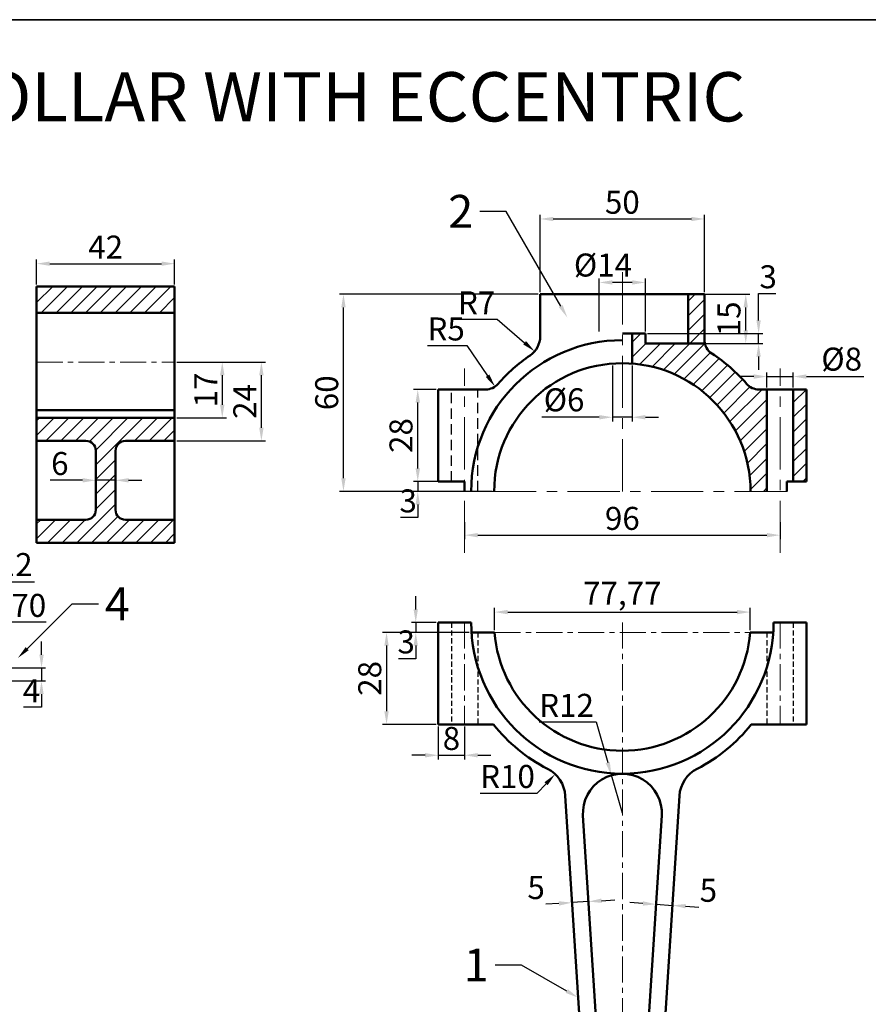
# Model space of a CAD drawing. Units: millimetres. Extents: x 214 to 813, y -258 to 321.
# Tile 3 of 4: x 416 to 674, y 22 to 321. Entities that reach past the tile are written whole.
import ezdxf
from ezdxf import colors
from ezdxf.entities.mleader import LeaderData, LeaderLine
from ezdxf.math import Vec2, Vec3

# ---------------------------------------------------------------- set-up
doc = ezdxf.new("R2010")
doc.units = ezdxf.units.MM
doc.header["$LTSCALE"] = 0.5
doc.linetypes.add('CENTER', pattern=[50.8, 31.75, -6.35, 6.35, -6.35])
doc.linetypes.add('HIDDEN', pattern=[9.525, 6.35, -3.175])
for name, color, linetype, lineweight in [('M-CNTR', 1, 'CENTER', 18), ('M-DIMS', 2, 'Continuous', 25), ('M-HATC', 8, 'Continuous', 18), ('M-HIDN', 6, 'HIDDEN', 25), ('M-OUTL', 7, 'Continuous', 50), ('M-TTLB', 7, 'Continuous', 35)]:
    doc.layers.add(name, color=color, linetype=linetype, lineweight=lineweight)
doc.styles.get("Standard").update_dxf_attribs({"font": 'arial.ttf'})
doc.dimstyles.new('ISO-25', dxfattribs={"dimtxt": 7, "dimasz": 4, "dimexe": 1.25, "dimexo": 0.625, "dimtad": 1, "dimtoh": 1, "dimtxsty": 'Standard', "dimcen": 2.5, "dimadec": 0, "dimazin": 0, "dimtfac": 1, "dimtmove": 0, "dimatfit": 3, "dimfxl": 1, "dimarcsym": 0})

# ---------------------------------------------------------------- blocks, each defined once
blk = doc.blocks.new('*D3')
at = {"layer": 'Defpoints', "color": 0, "ltscale": 0.5, "transparency": 16777216}
for p in [(624.66, 260.85), (574.66, 237.96), (624.66, 237.96)]:
    blk.add_point(p, dxfattribs=at)
at = {"layer": 'M-DIMS', "color": 0, "lineweight": -2, "ltscale": 0.5, "transparency": 16777216}
for p, q in [((574.66, 238.59), (574.66, 262.1)), ((578.66, 260.85), (620.66, 260.85)), ((624.66, 238.59), (624.66, 262.1))]:
    blk.add_line(p, q, dxfattribs=at)
at = {"layer": 'M-DIMS', "color": 0, "ltscale": 0.5, "transparency": 16777216}
for points in [[(578.66, 261.51), (578.66, 260.18), (574.66, 260.85)], [(620.66, 261.51), (620.66, 260.18), (624.66, 260.85)]]:
    blk.add_solid(points, dxfattribs=at)
at = {"layer": 'M-DIMS', "color": 0, "ltscale": 0.5, "transparency": 16777216, "insert": (599.66, 265.04), "char_height": 7, "attachment_point": 5}
blk.add_mtext('50', dxfattribs=at)
blk = doc.blocks.new('*D4')
at = {"layer": 'Defpoints', "color": 0, "ltscale": 0.5, "transparency": 16777216}
for p in [(592.66, 241.53), (592.66, 225.96), (606.66, 225.96)]:
    blk.add_point(p, dxfattribs=at)
at = {"layer": 'M-DIMS', "color": 0, "lineweight": -2, "ltscale": 0.5, "transparency": 16777216}
for p, q in [((592.66, 226.59), (592.66, 242.78)), ((606.66, 226.59), (606.66, 242.78)), ((602.66, 241.53), (596.66, 241.53))]:
    blk.add_line(p, q, dxfattribs=at)
at = {"layer": 'M-DIMS', "color": 0, "ltscale": 0.5, "transparency": 16777216}
for points in [[(596.66, 242.2), (596.66, 240.87), (592.66, 241.53)], [(602.66, 242.2), (602.66, 240.87), (606.66, 241.53)]]:
    blk.add_solid(points, dxfattribs=at)
at = {"layer": 'M-DIMS', "color": 0, "ltscale": 0.5, "transparency": 16777216, "insert": (593.76, 245.93), "char_height": 7, "attachment_point": 5}
blk.add_mtext('%%C14', dxfattribs=at)
blk = doc.blocks.new('*D5')
at = {"layer": 'Defpoints', "color": 0, "ltscale": 0.5, "transparency": 16777216}
for p in [(606.66, 225.96), (641.12, 225.96), (606.66, 222.96)]:
    blk.add_point(p, dxfattribs=at)
at = {"layer": 'M-DIMS', "color": 0, "lineweight": -2, "ltscale": 0.5, "transparency": 16777216}
for p, q in [((641.12, 229.96), (641.12, 238.16)), ((641.12, 238.16), (646.32, 238.16)), ((607.29, 225.96), (642.37, 225.96)), ((641.12, 222.96), (641.12, 225.96)), ((607.29, 222.96), (642.37, 222.96)), ((641.12, 218.96), (641.12, 214.96))]:
    blk.add_line(p, q, dxfattribs=at)
at = {"layer": 'M-DIMS', "color": 0, "ltscale": 0.5, "transparency": 16777216}
for points in [[(640.45, 229.96), (641.78, 229.96), (641.12, 225.96)], [(640.45, 218.96), (641.78, 218.96), (641.12, 222.96)]]:
    blk.add_solid(points, dxfattribs=at)
at = {"layer": 'M-DIMS', "color": 0, "ltscale": 0.5, "transparency": 16777216, "insert": (644.03, 242.36), "char_height": 7, "attachment_point": 5}
blk.add_mtext('3', dxfattribs=at)
blk = doc.blocks.new('*D6')
at = {"layer": 'Defpoints', "color": 0, "ltscale": 0.5, "transparency": 16777216}
for p in [(614.78, 237.96), (637.21, 237.96), (614.78, 222.96)]:
    blk.add_point(p, dxfattribs=at)
at = {"layer": 'M-DIMS', "color": 0, "lineweight": -2, "ltscale": 0.5, "transparency": 16777216}
for p, q in [((615.41, 237.96), (638.46, 237.96)), ((637.21, 226.96), (637.21, 233.96)), ((615.41, 222.96), (638.46, 222.96))]:
    blk.add_line(p, q, dxfattribs=at)
at = {"layer": 'M-DIMS', "color": 0, "ltscale": 0.5, "transparency": 16777216}
for points in [[(636.55, 233.96), (637.88, 233.96), (637.21, 237.96)], [(636.55, 226.96), (637.88, 226.96), (637.21, 222.96)]]:
    blk.add_solid(points, dxfattribs=at)
at = {"layer": 'M-DIMS', "color": 0, "ltscale": 0.5, "transparency": 16777216, "insert": (633.01, 230.46), "char_height": 7, "attachment_point": 5, "rotation": 90}
blk.add_mtext('15', dxfattribs=at)
blk = doc.blocks.new('*D7')
at = {"layer": 'Defpoints', "color": 0, "ltscale": 0.5, "transparency": 16777216}
for p in [(651.66, 212.9), (643.66, 208.96), (651.66, 208.96)]:
    blk.add_point(p, dxfattribs=at)
at = {"layer": 'M-DIMS', "color": 0, "lineweight": -2, "ltscale": 0.5, "transparency": 16777216}
for p, q in [((639.66, 212.9), (635.66, 212.9)), ((643.66, 209.59), (643.66, 214.15)), ((643.66, 212.9), (651.66, 212.9)), ((651.66, 209.59), (651.66, 214.15)), ((655.66, 212.9), (673.13, 212.9))]:
    blk.add_line(p, q, dxfattribs=at)
at = {"layer": 'M-DIMS', "color": 0, "ltscale": 0.5, "transparency": 16777216}
for points in [[(639.66, 213.56), (639.66, 212.23), (643.66, 212.9)], [(655.66, 213.56), (655.66, 212.23), (651.66, 212.9)]]:
    blk.add_solid(points, dxfattribs=at)
at = {"layer": 'M-DIMS', "color": 0, "ltscale": 0.5, "transparency": 16777216, "insert": (666.4, 217.29), "char_height": 7, "attachment_point": 5}
blk.add_mtext('%%C8', dxfattribs=at)
blk = doc.blocks.new('*D8')
at = {"layer": 'Defpoints', "color": 0, "ltscale": 0.5, "transparency": 16777216}
for p in [(514.81, 237.96), (574.66, 237.96), (560.66, 177.96)]:
    blk.add_point(p, dxfattribs=at)
at = {"layer": 'M-DIMS', "color": 0, "lineweight": -2, "ltscale": 0.5, "transparency": 16777216}
for p, q in [((574.04, 237.96), (513.56, 237.96)), ((514.81, 181.96), (514.81, 233.96)), ((560.04, 177.96), (513.56, 177.96))]:
    blk.add_line(p, q, dxfattribs=at)
at = {"layer": 'M-DIMS', "color": 0, "ltscale": 0.5, "transparency": 16777216}
for points in [[(514.15, 233.96), (515.48, 233.96), (514.81, 237.96)], [(514.15, 181.96), (515.48, 181.96), (514.81, 177.96)]]:
    blk.add_solid(points, dxfattribs=at)
at = {"layer": 'M-DIMS', "color": 0, "ltscale": 0.5, "transparency": 16777216, "insert": (510.62, 207.96), "char_height": 7, "attachment_point": 5, "rotation": 90}
blk.add_mtext('60', dxfattribs=at)
blk = doc.blocks.new('*D9')
at = {"layer": 'Defpoints', "color": 0, "ltscale": 0.5, "transparency": 16777216}
for p in [(537.42, 208.96), (543.66, 208.96), (543.66, 180.96)]:
    blk.add_point(p, dxfattribs=at)
at = {"layer": 'M-DIMS', "color": 0, "lineweight": -2, "ltscale": 0.5, "transparency": 16777216}
for p, q in [((543.04, 208.96), (536.17, 208.96)), ((537.42, 184.96), (537.42, 204.96)), ((543.04, 180.96), (536.17, 180.96))]:
    blk.add_line(p, q, dxfattribs=at)
at = {"layer": 'M-DIMS', "color": 0, "ltscale": 0.5, "transparency": 16777216}
for points in [[(536.75, 204.96), (538.09, 204.96), (537.42, 208.96)], [(536.75, 184.96), (538.09, 184.96), (537.42, 180.96)]]:
    blk.add_solid(points, dxfattribs=at)
at = {"layer": 'M-DIMS', "color": 0, "ltscale": 0.5, "transparency": 16777216, "insert": (533.22, 194.96), "char_height": 7, "attachment_point": 5, "rotation": 90}
blk.add_mtext('28', dxfattribs=at)
blk = doc.blocks.new('*D10')
at = {"layer": 'Defpoints', "color": 0, "ltscale": 0.5, "transparency": 16777216}
for p in [(547.66, 180.96), (537.42, 177.96), (547.66, 177.96)]:
    blk.add_point(p, dxfattribs=at)
at = {"layer": 'M-DIMS', "color": 0, "lineweight": -2, "ltscale": 0.5, "transparency": 16777216}
for p, q in [((537.42, 184.96), (537.42, 188.96)), ((547.04, 180.96), (536.17, 180.96)), ((537.42, 180.96), (537.42, 177.96)), ((547.04, 177.96), (536.17, 177.96)), ((537.42, 173.96), (537.42, 169.96)), ((537.42, 169.96), (532.21, 169.96))]:
    blk.add_line(p, q, dxfattribs=at)
at = {"layer": 'M-DIMS', "color": 0, "ltscale": 0.5, "transparency": 16777216}
for points in [[(536.75, 184.96), (538.09, 184.96), (537.42, 180.96)], [(536.75, 173.96), (538.09, 173.96), (537.42, 177.96)]]:
    blk.add_solid(points, dxfattribs=at)
at = {"layer": 'M-DIMS', "color": 0, "ltscale": 0.5, "transparency": 16777216, "insert": (534.5, 174.16), "char_height": 7, "attachment_point": 5}
blk.add_mtext('3', dxfattribs=at)
blk = doc.blocks.new('*D11')
at = {"layer": 'Defpoints', "color": 0, "ltscale": 0.5, "transparency": 16777216}
for p in [(596.66, 216.85), (602.66, 216.85), (596.66, 200.51)]:
    blk.add_point(p, dxfattribs=at)
at = {"layer": 'M-DIMS', "color": 0, "lineweight": -2, "ltscale": 0.5, "transparency": 16777216}
for p, q in [((596.66, 216.22), (596.66, 199.26)), ((602.66, 216.22), (602.66, 199.26)), ((592.66, 200.51), (575.21, 200.51)), ((602.66, 200.51), (596.66, 200.51)), ((606.66, 200.51), (610.66, 200.51))]:
    blk.add_line(p, q, dxfattribs=at)
at = {"layer": 'M-DIMS', "color": 0, "ltscale": 0.5, "transparency": 16777216}
for points in [[(592.66, 201.18), (592.66, 199.85), (596.66, 200.51)], [(606.66, 201.18), (606.66, 199.85), (602.66, 200.51)]]:
    blk.add_solid(points, dxfattribs=at)
at = {"layer": 'M-DIMS', "color": 0, "ltscale": 0.5, "transparency": 16777216, "insert": (581.94, 204.91), "char_height": 7, "attachment_point": 5}
blk.add_mtext('%%C6', dxfattribs=at)
blk = doc.blocks.new('*D12')
at = {"layer": 'Defpoints', "color": 0, "ltscale": 0.5, "transparency": 16777216}
for p in [(558.08, 213.96), (560.92, 209.84)]:
    blk.add_point(p, dxfattribs=at)
at = {"layer": 'M-DIMS', "color": 0, "lineweight": -2, "ltscale": 0.5, "transparency": 16777216}
for p, q in [((540.38, 222.3), (552.35, 222.3)), ((552.35, 222.3), (558.65, 213.14))]:
    blk.add_line(p, q, dxfattribs=at)
at = {"layer": 'M-DIMS', "color": 0, "ltscale": 0.5, "transparency": 16777216}
blk.add_solid([(559.2, 213.52), (558.1, 212.76), (560.92, 209.84)], dxfattribs=at)
at = {"layer": 'M-DIMS', "color": 0, "ltscale": 0.5, "transparency": 16777216, "insert": (546.05, 226.48), "char_height": 7, "attachment_point": 5}
blk.add_mtext('R5', dxfattribs=at)
blk = doc.blocks.new('*D13')
at = {"layer": 'Defpoints', "color": 0, "ltscale": 0.5, "transparency": 16777216}
for p in [(567.66, 225.13), (572.98, 220.58)]:
    blk.add_point(p, dxfattribs=at)
at = {"layer": 'M-DIMS', "color": 0, "lineweight": -2, "ltscale": 0.5, "transparency": 16777216}
for p, q in [((549.68, 230.34), (561.59, 230.34)), ((561.59, 230.34), (569.94, 223.18))]:
    blk.add_line(p, q, dxfattribs=at)
at = {"layer": 'M-DIMS', "color": 0, "ltscale": 0.5, "transparency": 16777216}
blk.add_solid([(570.38, 223.69), (569.51, 222.67), (572.98, 220.58)], dxfattribs=at)
at = {"layer": 'M-DIMS', "color": 0, "ltscale": 0.5, "transparency": 16777216, "insert": (555.32, 234.46), "char_height": 7, "attachment_point": 5}
blk.add_mtext('R7', dxfattribs=at)
blk = doc.blocks.new('*D14')
at = {"layer": 'Defpoints', "color": 0, "ltscale": 0.5, "transparency": 16777216}
for p in [(551.66, 169.21), (647.66, 169.21), (647.66, 164.63)]:
    blk.add_point(p, dxfattribs=at)
at = {"layer": 'M-DIMS', "color": 0, "lineweight": -2, "ltscale": 0.5, "transparency": 16777216}
for p, q in [((551.66, 168.59), (551.66, 163.38)), ((647.66, 168.59), (647.66, 163.38)), ((555.66, 164.63), (643.66, 164.63))]:
    blk.add_line(p, q, dxfattribs=at)
at = {"layer": 'M-DIMS', "color": 0, "ltscale": 0.5, "transparency": 16777216}
for points in [[(555.66, 165.3), (555.66, 163.96), (551.66, 164.63)], [(643.66, 165.3), (643.66, 163.96), (647.66, 164.63)]]:
    blk.add_solid(points, dxfattribs=at)
at = {"layer": 'M-DIMS', "color": 0, "ltscale": 0.5, "transparency": 16777216, "insert": (599.66, 168.83), "char_height": 7, "attachment_point": 5}
blk.add_mtext('96', dxfattribs=at)
blk = doc.blocks.new('*D15')
at = {"layer": 'Defpoints', "color": 0, "ltscale": 0.5, "transparency": 16777216}
for p in [(543.66, 138.04), (536.81, 135.04), (553.66, 135.04)]:
    blk.add_point(p, dxfattribs=at)
at = {"layer": 'M-DIMS', "color": 0, "lineweight": -2, "ltscale": 0.5, "transparency": 16777216}
for p, q in [((536.81, 142.04), (536.81, 146.04)), ((543.04, 138.04), (535.56, 138.04)), ((536.81, 138.04), (536.81, 135.04)), ((553.04, 135.04), (535.56, 135.04)), ((536.81, 131.04), (536.81, 127.04)), ((536.81, 127.04), (531.6, 127.04))]:
    blk.add_line(p, q, dxfattribs=at)
at = {"layer": 'M-DIMS', "color": 0, "ltscale": 0.5, "transparency": 16777216}
for points in [[(536.14, 142.04), (537.47, 142.04), (536.81, 138.04)], [(536.14, 131.04), (537.47, 131.04), (536.81, 135.04)]]:
    blk.add_solid(points, dxfattribs=at)
at = {"layer": 'M-DIMS', "color": 0, "ltscale": 0.5, "transparency": 16777216, "insert": (533.89, 131.24), "char_height": 7, "attachment_point": 5}
blk.add_mtext('3', dxfattribs=at)
blk = doc.blocks.new('*D16')
at = {"layer": 'Defpoints', "color": 0, "ltscale": 0.5, "transparency": 16777216}
for p in [(543.66, 135.04), (527.92, 107.04), (543.66, 107.04)]:
    blk.add_point(p, dxfattribs=at)
at = {"layer": 'M-DIMS', "color": 0, "lineweight": -2, "ltscale": 0.5, "transparency": 16777216}
for p, q in [((543.04, 135.04), (526.67, 135.04)), ((527.92, 131.04), (527.92, 111.04)), ((543.04, 107.04), (526.67, 107.04))]:
    blk.add_line(p, q, dxfattribs=at)
at = {"layer": 'M-DIMS', "color": 0, "ltscale": 0.5, "transparency": 16777216}
for points in [[(527.25, 131.04), (528.58, 131.04), (527.92, 135.04)], [(527.25, 111.04), (528.58, 111.04), (527.92, 107.04)]]:
    blk.add_solid(points, dxfattribs=at)
at = {"layer": 'M-DIMS', "color": 0, "ltscale": 0.5, "transparency": 16777216, "insert": (523.72, 121.04), "char_height": 7, "attachment_point": 5, "rotation": 90}
blk.add_mtext('28', dxfattribs=at)
blk = doc.blocks.new('*D17')
at = {"layer": 'Defpoints', "color": 0, "ltscale": 0.5, "transparency": 16777216}
for p in [(543.66, 107.04), (551.66, 107.04), (551.66, 97.65)]:
    blk.add_point(p, dxfattribs=at)
at = {"layer": 'M-DIMS', "color": 0, "lineweight": -2, "ltscale": 0.5, "transparency": 16777216}
for p, q in [((543.66, 106.42), (543.66, 96.4)), ((551.66, 106.42), (551.66, 96.4)), ((539.66, 97.65), (535.66, 97.65)), ((543.66, 97.65), (551.66, 97.65)), ((555.66, 97.65), (559.66, 97.65))]:
    blk.add_line(p, q, dxfattribs=at)
at = {"layer": 'M-DIMS', "color": 0, "ltscale": 0.5, "transparency": 16777216}
for points in [[(539.66, 98.32), (539.66, 96.98), (543.66, 97.65)], [(555.66, 98.32), (555.66, 96.98), (551.66, 97.65)]]:
    blk.add_solid(points, dxfattribs=at)
at = {"layer": 'M-DIMS', "color": 0, "ltscale": 0.5, "transparency": 16777216, "insert": (547.66, 101.85), "char_height": 7, "attachment_point": 5}
blk.add_mtext('8', dxfattribs=at)
blk = doc.blocks.new('*D18')
at = {"layer": 'Defpoints', "color": 0, "ltscale": 0.5, "transparency": 16777216}
for p in [(638.55, 141.22), (560.78, 135.04), (638.55, 135.04)]:
    blk.add_point(p, dxfattribs=at)
at = {"layer": 'M-DIMS', "color": 0, "lineweight": -2, "ltscale": 0.5, "transparency": 16777216}
for p, q in [((560.78, 135.67), (560.78, 142.47)), ((564.78, 141.22), (634.55, 141.22)), ((638.55, 135.67), (638.55, 142.47))]:
    blk.add_line(p, q, dxfattribs=at)
at = {"layer": 'M-DIMS', "color": 0, "ltscale": 0.5, "transparency": 16777216}
for points in [[(564.78, 141.89), (564.78, 140.56), (560.78, 141.22)], [(634.55, 141.89), (634.55, 140.56), (638.55, 141.22)]]:
    blk.add_solid(points, dxfattribs=at)
at = {"layer": 'M-DIMS', "color": 0, "ltscale": 0.5, "transparency": 16777216, "insert": (599.66, 146.04), "char_height": 7, "attachment_point": 5}
blk.add_mtext('77,77', dxfattribs=at)
blk = doc.blocks.new('*D19')
at = {"layer": 'Defpoints', "color": 0, "ltscale": 0.5, "transparency": 16777216}
for p in [(579.21, 91.88), (572.32, 84.64)]:
    blk.add_point(p, dxfattribs=at)
at = {"layer": 'M-DIMS', "color": 0, "lineweight": -2, "ltscale": 0.5, "transparency": 16777216}
for p, q in [((573.7, 86.09), (576.45, 88.99)), ((556.37, 86.09), (573.7, 86.09))]:
    blk.add_line(p, q, dxfattribs=at)
at = {"layer": 'M-DIMS', "color": 0, "ltscale": 0.5, "transparency": 16777216}
blk.add_solid([(575.97, 89.44), (576.93, 88.53), (579.21, 91.88)], dxfattribs=at)
at = {"layer": 'M-DIMS', "color": 0, "ltscale": 0.5, "transparency": 16777216, "insert": (564.72, 90.29), "char_height": 7, "attachment_point": 5}
blk.add_mtext('R10', dxfattribs=at)
blk = doc.blocks.new('*D20')
at = {"layer": 'Defpoints', "color": 0, "ltscale": 0.5, "transparency": 16777216}
for p in [(596.33, 91.57), (599.66, 80.04)]:
    blk.add_point(p, dxfattribs=at)
at = {"layer": 'M-DIMS', "color": 0, "lineweight": -2, "ltscale": 0.5, "transparency": 16777216}
for p, q in [((574.37, 107.79), (591.65, 107.79)), ((591.65, 107.79), (595.22, 95.41)), ((599.66, 80.04), (596.33, 91.57))]:
    blk.add_line(p, q, dxfattribs=at)
at = {"layer": 'M-DIMS', "color": 0, "ltscale": 0.5, "transparency": 16777216}
blk.add_solid([(595.86, 95.6), (594.58, 95.23), (596.33, 91.57)], dxfattribs=at)
at = {"layer": 'M-DIMS', "color": 0, "ltscale": 0.5, "transparency": 16777216, "insert": (582.69, 111.93), "char_height": 7, "attachment_point": 5}
blk.add_mtext('R12', dxfattribs=at)
blk = doc.blocks.new('*D21')
at = {"layer": 'Defpoints', "color": 0, "ltscale": 0.5, "transparency": 16777216}
for p in [(584.35, 53), (589.34, 53.31), (589.35, 53.13)]:
    blk.add_point(p, dxfattribs=at)
at = {"layer": 'M-DIMS', "color": 0, "lineweight": -2, "ltscale": 0.5, "transparency": 16777216}
for p, q in [((580.37, 52.56), (576.38, 52.3)), ((589.35, 53.13), (584.36, 52.81)), ((584.39, 52.37), (584.44, 51.56)), ((589.38, 52.69), (589.43, 51.88)), ((593.34, 53.38), (597.34, 53.64))]:
    blk.add_line(p, q, dxfattribs=at)
at = {"layer": 'M-DIMS', "color": 0, "ltscale": 0.5, "transparency": 16777216}
for points in [[(593.3, 54.05), (593.39, 52.72), (589.35, 53.13)], [(580.33, 53.22), (580.41, 51.89), (584.36, 52.81)]]:
    blk.add_solid(points, dxfattribs=at)
at = {"layer": 'M-DIMS', "color": 0, "ltscale": 0.5, "transparency": 16777216, "insert": (573.43, 56.49), "char_height": 7, "attachment_point": 5}
blk.add_mtext('5', dxfattribs=at)
blk = doc.blocks.new('*D22')
at = {"layer": 'Defpoints', "color": 0, "ltscale": 0.5, "transparency": 16777216}
for p in [(614.91, 51.97), (609.64, 47.91), (614.63, 47.59)]:
    blk.add_point(p, dxfattribs=at)
at = {"layer": 'M-DIMS', "color": 0, "lineweight": -2, "ltscale": 0.5, "transparency": 16777216}
for p, q in [((605.93, 52.54), (601.94, 52.8)), ((609.68, 48.53), (610, 53.54)), ((609.92, 52.29), (614.91, 51.97)), ((614.67, 48.21), (614.99, 53.22)), ((618.9, 51.72), (622.9, 51.46))]:
    blk.add_line(p, q, dxfattribs=at)
at = {"layer": 'M-DIMS', "color": 0, "ltscale": 0.5, "transparency": 16777216}
for points in [[(605.97, 53.21), (605.89, 51.88), (609.92, 52.29)], [(618.95, 52.38), (618.86, 51.05), (614.91, 51.97)]]:
    blk.add_solid(points, dxfattribs=at)
at = {"layer": 'M-DIMS', "color": 0, "ltscale": 0.5, "transparency": 16777216, "insert": (625.84, 55.65), "char_height": 7, "attachment_point": 5}
blk.add_mtext('5', dxfattribs=at)
blk = doc.blocks.new('*D33')
at = {"layer": 'Defpoints', "color": 0, "ltscale": 0.5, "transparency": 16777216}
for p in [(463.45, 247.25), (421.45, 240.32), (463.45, 240.32)]:
    blk.add_point(p, dxfattribs=at)
at = {"layer": 'M-DIMS', "color": 0, "lineweight": -2, "ltscale": 0.5, "transparency": 16777216}
for p, q in [((421.45, 240.95), (421.45, 248.5)), ((425.45, 247.25), (459.45, 247.25)), ((463.45, 240.95), (463.45, 248.5))]:
    blk.add_line(p, q, dxfattribs=at)
at = {"layer": 'M-DIMS', "color": 0, "ltscale": 0.5, "transparency": 16777216}
for points in [[(425.45, 247.92), (425.45, 246.58), (421.45, 247.25)], [(459.45, 247.92), (459.45, 246.58), (463.45, 247.25)]]:
    blk.add_solid(points, dxfattribs=at)
at = {"layer": 'M-DIMS', "color": 0, "ltscale": 0.5, "transparency": 16777216, "insert": (442.45, 251.39), "char_height": 7, "attachment_point": 5}
blk.add_mtext('42', dxfattribs=at)
blk = doc.blocks.new('*D34')
at = {"layer": 'Defpoints', "color": 0, "ltscale": 0.5, "transparency": 16777216}
for p in [(463.45, 217.32), (463.45, 200.32), (477.94, 200.32)]:
    blk.add_point(p, dxfattribs=at)
at = {"layer": 'M-DIMS', "color": 0, "lineweight": -2, "ltscale": 0.5, "transparency": 16777216}
for p, q in [((464.08, 217.32), (479.19, 217.32)), ((477.94, 213.32), (477.94, 204.32)), ((464.08, 200.32), (479.19, 200.32))]:
    blk.add_line(p, q, dxfattribs=at)
at = {"layer": 'M-DIMS', "color": 0, "ltscale": 0.5, "transparency": 16777216}
for points in [[(477.27, 213.32), (478.6, 213.32), (477.94, 217.32)], [(477.27, 204.32), (478.6, 204.32), (477.94, 200.32)]]:
    blk.add_solid(points, dxfattribs=at)
at = {"layer": 'M-DIMS', "color": 0, "ltscale": 0.5, "transparency": 16777216, "insert": (473.8, 208.82), "char_height": 7, "attachment_point": 5, "rotation": 90}
blk.add_mtext('17', dxfattribs=at)
blk = doc.blocks.new('*D35')
at = {"layer": 'Defpoints', "color": 0, "ltscale": 0.5, "transparency": 16777216}
for p in [(463.45, 217.32), (489.84, 217.32), (463.45, 193.32)]:
    blk.add_point(p, dxfattribs=at)
at = {"layer": 'M-DIMS', "color": 0, "lineweight": -2, "ltscale": 0.5, "transparency": 16777216}
for p, q in [((464.08, 217.32), (491.09, 217.32)), ((489.84, 197.32), (489.84, 213.32)), ((464.08, 193.32), (491.09, 193.32))]:
    blk.add_line(p, q, dxfattribs=at)
at = {"layer": 'M-DIMS', "color": 0, "ltscale": 0.5, "transparency": 16777216}
for points in [[(489.17, 213.32), (490.51, 213.32), (489.84, 217.32)], [(489.17, 197.32), (490.51, 197.32), (489.84, 193.32)]]:
    blk.add_solid(points, dxfattribs=at)
at = {"layer": 'M-DIMS', "color": 0, "ltscale": 0.5, "transparency": 16777216, "insert": (485.7, 205.32), "char_height": 7, "attachment_point": 5, "rotation": 90}
blk.add_mtext('24', dxfattribs=at)
blk = doc.blocks.new('*D36')
at = {"layer": 'Defpoints', "color": 0, "ltscale": 0.5, "transparency": 16777216}
for p in [(439.45, 181.32), (445.45, 181.32), (445.45, 181.32)]:
    blk.add_point(p, dxfattribs=at)
at = {"layer": 'M-DIMS', "color": 0, "lineweight": -2, "ltscale": 0.5, "transparency": 16777216}
for p, q in [((435.45, 181.32), (425.58, 181.32)), ((439.45, 181.95), (439.45, 182.57)), ((445.45, 181.32), (439.45, 181.32)), ((445.45, 181.95), (445.45, 182.57)), ((449.45, 181.32), (453.45, 181.32))]:
    blk.add_line(p, q, dxfattribs=at)
at = {"layer": 'M-DIMS', "color": 0, "ltscale": 0.5, "transparency": 16777216}
for points in [[(435.45, 181.99), (435.45, 180.66), (439.45, 181.32)], [(449.45, 181.99), (449.45, 180.66), (445.45, 181.32)]]:
    blk.add_solid(points, dxfattribs=at)
at = {"layer": 'M-DIMS', "color": 0, "ltscale": 0.5, "transparency": 16777216, "insert": (428.52, 185.52), "char_height": 7, "attachment_point": 5}
blk.add_mtext('6', dxfattribs=at)
blk = doc.blocks.new('*D47')
at = {"layer": 'Defpoints', "color": 0, "ltscale": 0.5, "transparency": 16777216}
for p in [(396.75, 150.39), (384.75, 134.26), (396.75, 134.26)]:
    blk.add_point(p, dxfattribs=at)
at = {"layer": 'M-DIMS', "color": 0, "lineweight": -2, "ltscale": 0.5, "transparency": 16777216}
for p, q in [((384.75, 134.88), (384.75, 151.64)), ((388.75, 150.39), (392.75, 150.39)), ((396.75, 134.88), (396.75, 151.64)), ((396.75, 150.39), (420.79, 150.39))]:
    blk.add_line(p, q, dxfattribs=at)
at = {"layer": 'M-DIMS', "color": 0, "ltscale": 0.5, "transparency": 16777216}
for points in [[(388.75, 151.05), (388.75, 149.72), (384.75, 150.39)], [(392.75, 151.05), (392.75, 149.72), (396.75, 150.39)]]:
    blk.add_solid(points, dxfattribs=at)
at = {"layer": 'M-DIMS', "color": 0, "ltscale": 0.5, "transparency": 16777216, "insert": (411.38, 154.78), "char_height": 7, "attachment_point": 5}
blk.add_mtext('%%C12', dxfattribs=at)
blk = doc.blocks.new('*D53')
at = {"layer": 'Defpoints', "color": 0, "ltscale": 0.5, "transparency": 16777216}
for p in [(410.75, 124.26), (410.75, 120.26), (422.94, 120.26)]:
    blk.add_point(p, dxfattribs=at)
at = {"layer": 'M-DIMS', "color": 0, "lineweight": -2, "ltscale": 0.5, "transparency": 16777216}
for p, q in [((422.94, 128.26), (422.94, 132.26)), ((411.37, 124.26), (424.19, 124.26)), ((422.94, 124.26), (422.94, 120.26)), ((411.37, 120.26), (424.19, 120.26)), ((422.94, 116.26), (422.94, 112.26)), ((422.94, 112.26), (417.48, 112.26))]:
    blk.add_line(p, q, dxfattribs=at)
at = {"layer": 'M-DIMS', "color": 0, "ltscale": 0.5, "transparency": 16777216}
for points in [[(422.28, 128.26), (423.61, 128.26), (422.94, 124.26)], [(422.28, 116.26), (423.61, 116.26), (422.94, 120.26)]]:
    blk.add_solid(points, dxfattribs=at)
at = {"layer": 'M-DIMS', "color": 0, "ltscale": 0.5, "transparency": 16777216, "insert": (419.9, 116.38), "char_height": 7, "attachment_point": 5}
blk.add_mtext('4', dxfattribs=at)
blk = doc.blocks.new('*D55')
at = {"layer": 'Defpoints', "color": 0, "ltscale": 0.5, "transparency": 16777216}
for p in [(405.38, 130.33), (390.75, 61.88)]:
    blk.add_point(p, dxfattribs=at)
at = {"layer": 'M-DIMS', "color": 0, "lineweight": -2, "ltscale": 0.5, "transparency": 16777216}
for p, q in [((407.06, 138.15), (406.22, 134.24)), ((424.38, 138.15), (407.06, 138.15)), ((390.75, 61.88), (405.38, 130.33))]:
    blk.add_line(p, q, dxfattribs=at)
at = {"layer": 'M-DIMS', "color": 0, "ltscale": 0.5, "transparency": 16777216}
blk.add_solid([(405.57, 134.38), (406.87, 134.1), (405.38, 130.33)], dxfattribs=at)
at = {"layer": 'M-DIMS', "color": 0, "ltscale": 0.5, "transparency": 16777216, "insert": (416.03, 142.35), "char_height": 7, "attachment_point": 5}
blk.add_mtext('R70', dxfattribs=at)

msp = doc.modelspace()

# ---------------------------------------------------------------- hatches: boundary and pattern name
at = {"layer": 'M-HATC', "ltscale": 0.5}
h = msp.add_hatch(dxfattribs=at)
h.set_pattern_fill('ANSI31', color=256)
h.set_pattern_definition([(45, (63.6263, 88.602), (-2.245064, 2.245064), [])])
h.paths.add_polyline_path([(463.452, 232.322), (463.452, 240.322), (421.452, 240.322), (421.452, 232.322)])
h.paths.add_polyline_path([(421.452, 200.322), (421.452, 193.322), (436.452, 193.322, -0.4142136), (439.452, 190.322), (439.452, 172.322, -0.4142136), (436.452, 169.322), (421.452, 169.322), (421.452, 162.322), (463.452, 162.322), (463.452, 169.322), (448.452, 169.322, -0.4142136), (445.452, 172.322), (445.452, 190.322, -0.4142136), (448.452, 193.322), (463.452, 193.322), (463.452, 200.322)])
h = msp.add_hatch(dxfattribs=at)
h.set_pattern_fill('ANSI31', color=256)
h.set_pattern_definition([(45, (455.661, 0), (-2.245064, 2.245064), [])])
h.paths.add_polyline_path([(624.664, 221.263), (624.664, 237.962), (619.664, 237.962), (619.664, 222.962), (606.664, 222.962), (606.664, 225.962), (602.664, 225.962), (602.664, 216.846, -0.3918367), (638.664, 177.962), (643.664, 177.962), (643.664, 208.962), (638.894, 208.962, 0.094897)])
h.paths.add_polyline_path([(655.664, 208.962), (651.664, 208.962), (651.664, 180.962), (655.664, 180.962)])

# ---------------------------------------------------------------- linework, layer by layer
at = {"layer": 'M-CNTR'}
for p, q in [((599.664, 177.962), (599.664, 245.711)), ((551.664, 159.243), (551.664, 215.306)), ((647.664, 159.243), (647.664, 215.306)), ((649.664, 177.962), (551.664, 177.962))]:
    msp.add_line(p, q, dxfattribs=at)
at = {"layer": 'M-CNTR', "ltscale": 0.5}
for p, q in [((421.452, 217.322), (463.452, 217.322)), ((551.664, 138.042), (551.664, 107.042)), ((599.664, 138.042), (599.664, -30.466)), ((647.664, 138.042), (647.664, 107.042)), ((560.78, 135.042), (638.549, 135.042))]:
    msp.add_line(p, q, dxfattribs=at)
at = {"layer": 'M-HIDN'}
for p, q in [((547.664, 180.962), (547.664, 208.962)), ((555.664, 177.962), (555.664, 208.962))]:
    msp.add_line(p, q, dxfattribs=at)
at = {"layer": 'M-HIDN', "ltscale": 0.5}
for p, q in [((547.664, 138.042), (547.664, 107.042)), ((651.664, 138.042), (651.664, 107.042)), ((555.664, 135.042), (555.664, 107.042)), ((643.664, 135.042), (643.664, 107.042))]:
    msp.add_line(p, q, dxfattribs=at)
at = {"layer": 'M-OUTL', "ltscale": 0.5}
for p, q in [((421.452, 240.322), (421.452, 162.322)), ((463.452, 240.322), (421.452, 240.322)), ((463.452, 162.322), (463.452, 240.322)), ((421.452, 232.322), (463.452, 232.322)), ((606.664, 222.962), (624.786, 222.962)), ((421.452, 202.625), (463.452, 202.625)), ((421.452, 200.322), (463.452, 200.322)), ((421.452, 193.322), (436.452, 193.322)), ((448.452, 193.322), (463.452, 193.322)), ((439.452, 190.322), (439.452, 172.322)), ((445.452, 190.322), (445.452, 172.322)), ((655.664, 180.962), (649.664, 180.962)), ((649.664, 177.962), (649.664, 180.962)), ((421.452, 169.322), (436.452, 169.322)), ((448.452, 169.322), (463.452, 169.322)), ((421.452, 162.322), (463.452, 162.322)), ((543.664, 138.042), (543.664, 107.042)), ((553.664, 138.042), (543.664, 138.042)), ((645.664, 138.042), (655.664, 138.042)), ((655.664, 138.042), (655.664, 107.042)), ((560.78, 135.042), (553.664, 135.042)), ((638.549, 135.042), (645.566, 135.042)), ((560.434, 107.042), (543.664, 107.042)), ((638.894, 107.042), (655.664, 107.042)), ((582.297, 85.272), (587.342, 5.974)), ((617.031, 85.272), (611.986, 5.974)), ((587.689, 79.28), (591.68, 16.534)), ((611.64, 79.28), (607.648, 16.534))]:
    msp.add_line(p, q, dxfattribs=at)
at = {"layer": 'M-OUTL'}
for p, q in [((574.664, 237.962), (624.664, 237.962)), ((574.664, 237.962), (574.664, 225.132)), ((619.664, 237.962), (619.664, 222.962)), ((624.664, 237.962), (624.664, 224.06)), ((606.664, 225.962), (599.664, 225.962)), ((602.664, 216.846), (602.664, 225.962)), ((606.664, 222.962), (606.664, 225.962)), ((619.664, 222.962), (606.664, 222.962)), ((543.664, 180.962), (543.664, 208.962)), ((558.083, 208.962), (543.664, 208.962)), ((641.246, 208.962), (655.664, 208.962)), ((643.664, 177.962), (643.664, 208.962)), ((651.664, 180.962), (651.664, 208.962)), ((655.664, 180.962), (655.664, 208.962)), ((551.664, 180.962), (543.664, 180.962)), ((551.664, 177.962), (551.664, 180.962))]:
    msp.add_line(p, q, dxfattribs=at)
for centre, radius, start, end in [((567.664, 225.132), 7, 304.15292, 0), ((599.664, 177.962), 46, 90, 180), ((629.664, 224.06), 5, 180, 236.94427), ((599.664, 177.962), 50, 124.15292, 139.11481), ((599.664, 177.962), 50, 40.88519, 56.94427), ((599.664, 177.962), 39, 0, 180), ((558.083, 213.962), 5, 270, 319.11481), ((641.246, 213.962), 5, 220.88519, 270)]:
    msp.add_arc(centre, radius, start, end, dxfattribs=at)
at = {"layer": 'M-OUTL', "ltscale": 0.5}
for centre, radius, start, end in [((436.452, 190.322), 3, 0, 90), ((448.452, 190.322), 3, 90, 180), ((436.452, 172.322), 3, 270, 0), ((448.452, 172.322), 3, 180, 270), ((599.664, 138.042), 46, 180, 0), ((599.664, 138.042), 39, 184.41173, 355.58827), ((599.664, 138.042), 50, 218.31613, 242.88477), ((599.664, 138.042), 50, 297.11523, 321.68387), ((572.317, 84.637), 10, 3.64028, 62.88477), ((627.011, 84.637), 10, 117.11523, 176.35972), ((599.664, 80.042), 12, 356.35972, 183.64028)]:
    msp.add_arc(centre, radius, start, end, dxfattribs=at)
at = {"layer": 'M-TTLB', "ltscale": 0.5}
msp.add_lwpolyline([(214.186, 321.5), (812.717, 321.5), (812.717, -258.089), (214.186, -258.089)], close=True, dxfattribs=at)

# ---------------------------------------------------------------- texts
at = {"layer": 'M-TTLB', "ltscale": 0.5, "insert": (391.608, 305.53), "char_height": 15, "attachment_point": 1}
msp.add_mtext_dynamic_manual_height_columns('COLLAR WITH ECCENTRIC ', width=324.14999, gutter_width=12.5, heights=[0], dxfattribs=at)

# ---------------------------------------------------------------- dimensions: what is measured, and where the dimension line sits
at = {"layer": 'M-DIMS', "ltscale": 0.5}
for base, p1, p2, picture, middle in [((624.664, 260.845), (574.664, 237.962), (624.664, 237.962), '*D3', (599.664, 265.044)), ((463.452, 247.251), (421.452, 240.322), (463.452, 240.322), '*D33', (442.452, 251.391)), ((647.664, 164.63), (551.664, 169.212), (647.664, 169.212), '*D14', (599.664, 168.829)), ((638.549, 141.223), (560.78, 135.042), (638.549, 135.042), '*D18', (599.664, 146.04))]:
    dim = msp.add_linear_dim(base=base, p1=p1, p2=p2, dimstyle='ISO-25', override={"dimclrd": 0, "dimclre": 0, "dimclrt": 0}, dxfattribs=at)
    dim.commit()
    dim.dimension.update_dxf_attribs({"geometry": picture, "text_midpoint": middle})
for base, p1, p2, picture, middle in [((592.664, 241.534), (606.664, 225.962), (592.664, 225.962), '*D4', (593.761, 241.534)), ((596.664, 200.512), (602.664, 216.846), (596.664, 216.846), '*D11', (581.939, 200.512)), ((396.748, 150.387), (384.748, 134.26), (396.748, 134.26), '*D47', (411.38, 150.387))]:
    dim = msp.add_linear_dim(base=base, p1=p1, p2=p2, text='%%C<>', dimstyle='ISO-25', override={"dimclrd": 0, "dimclre": 0, "dimclrt": 0}, dxfattribs=at)
    dim.commit()
    dim.dimension.update_dxf_attribs({"geometry": picture, "text_midpoint": middle, "dimtype": 160})
for base, p1, p2, angle, picture, middle, dimtype in [((641.115, 225.962), (606.664, 222.962), (606.664, 225.962), 90, '*D5', (644.032, 238.163), 160), ((589.352, 53.128), (584.351, 52.997), (589.341, 53.314), 3.64028, '*D21', (573.433, 52.302), 161)]:
    dim = msp.add_linear_dim(base=base, p1=p1, p2=p2, angle=angle, dimstyle='ISO-25', override={"dimclrd": 0, "dimclre": 0, "dimclrt": 0}, dxfattribs=at)
    dim.commit()
    dim.dimension.update_dxf_attribs({"geometry": picture, "text_midpoint": middle, "dimtype": dimtype})
for base, p1, p2, picture, middle in [((514.814, 237.962), (560.664, 177.962), (574.664, 237.962), '*D8', (510.615, 207.962)), ((637.212, 237.962), (614.784, 222.962), (614.784, 237.962), '*D6', (633.013, 230.462)), ((477.938, 200.322), (463.452, 217.322), (463.452, 200.322), '*D34', (473.799, 208.822)), ((489.84, 217.322), (463.452, 193.322), (463.452, 217.322), '*D35', (485.7, 205.322)), ((537.421, 208.962), (543.664, 180.962), (543.664, 208.962), '*D9', (533.222, 194.962)), ((537.421, 177.962), (547.664, 180.962), (547.664, 177.962), '*D10', (534.504, 174.163)), ((536.806, 135.042), (543.664, 138.042), (553.664, 135.042), '*D15', (533.889, 131.244)), ((527.916, 107.042), (543.664, 135.042), (543.664, 107.042), '*D16', (523.717, 121.042)), ((422.944, 120.26), (410.748, 124.26), (410.748, 120.26), '*D53', (419.898, 116.385))]:
    dim = msp.add_linear_dim(base=base, p1=p1, p2=p2, angle=90, dimstyle='ISO-25', override={"dimclrd": 0, "dimclre": 0, "dimclrt": 0}, dxfattribs=at)
    dim.commit()
    dim.dimension.update_dxf_attribs({"geometry": picture, "text_midpoint": middle})
for center, mpoint, picture, middle in [((567.664, 225.132), (572.979, 220.576), '*D13', (555.322, 230.338)), ((558.083, 213.962), (560.917, 209.843), '*D12', (546.052, 222.298)), ((599.664, 80.042), (596.333, 91.571), '*D20', (582.693, 107.79)), ((572.317, 84.637), (579.207, 91.885), '*D19', (564.719, 86.086))]:
    dim = msp.add_radius_dim(center=center, mpoint=mpoint, dimstyle='ISO-25', override={"dimclrd": 0, "dimclre": 0, "dimclrt": 0}, dxfattribs=at)
    dim.commit()
    dim.dimension.update_dxf_attribs({"geometry": picture, "text_midpoint": middle, "dimtype": 164})
dim = msp.add_linear_dim(base=(651.664, 212.896), p1=(643.664, 208.962), p2=(651.664, 208.962), text='%%C<>', dimstyle='ISO-25', override={"dimclrd": 0, "dimclre": 0, "dimclrt": 0}, dxfattribs=at)
dim.commit()
dim.dimension.update_dxf_attribs({"geometry": '*D7', "text_midpoint": (666.399, 217.291)})
for base, p1, p2, picture, middle in [((445.452, 181.322), (439.452, 181.322), (445.452, 181.322), '*D36', (428.516, 181.322)), ((551.664, 97.652), (543.664, 107.042), (551.664, 107.042), '*D17', (547.664, 97.652))]:
    dim = msp.add_linear_dim(base=base, p1=p1, p2=p2, dimstyle='ISO-25', override={"dimclrd": 0, "dimclre": 0, "dimclrt": 0}, dxfattribs=at)
    dim.commit()
    dim.dimension.update_dxf_attribs({"geometry": picture, "text_midpoint": middle, "dimtype": 160})
dim = msp.add_radius_dim(center=(390.748, 61.876), mpoint=(405.383, 130.329), dimstyle='ISO-25', override={"dimclrd": 0, "dimclre": 0, "dimclrt": 0}, dxfattribs=at)
dim.commit()
dim.dimension.update_dxf_attribs({"geometry": '*D55', "text_midpoint": (416.032, 142.351)})
dim = msp.add_aligned_dim(p1=(609.644, 47.907), p2=(614.634, 47.59), distance=4.389, dimstyle='ISO-25', override={"dimclrd": 0, "dimclre": 0, "dimclrt": 0}, dxfattribs=at)
dim.commit()
dim.dimension.update_dxf_attribs({"geometry": '*D22', "text_midpoint": (625.842, 55.647)})

# ---------------------------------------------------------------- leaders
ml = msp.add_multileader_mtext('Standard', dxfattribs=at)
ml.set_content('2', color=256)
ml.set_leader_properties()
ml.build(insert=Vec2(0, 0))
ctx = ml.context
ctx.base_point, ctx.char_height, ctx.plane_origin = Vec3(545.644, 263.174), 10, Vec3(582.924, 230.86)
ctx.text_align_type = 2
notes = []
notes.append((ctx, [(0, (1, 1, 0), (564.267, 263.174), (-1, 0), 8, [(0, [(582.924, 230.86)], 0, [])])]))
ctx.mtext.insert, ctx.mtext.alignment, ctx.mtext.flow_direction = Vec3(554.267, 268.174), 3, 5
ml = msp.add_multileader_mtext('Standard', dxfattribs=at)
ml.set_content('4', color=256)
ml.set_leader_properties()
ml.build(insert=Vec2(0, 0))
ctx = ml.context
ctx.base_point, ctx.char_height, ctx.plane_origin = Vec3(440.235, 143.705), 10, Vec3(415.748, 127.26)
notes.append((ctx, [(0, (1, 1, 0), (432.235, 143.705), (1, 0), 8, [(0, [(415.748, 127.26)], 0, [])])]))
ctx.mtext.insert, ctx.mtext.flow_direction = Vec3(442.235, 148.705), 5
ml = msp.add_multileader_mtext('Standard', dxfattribs=at)
ml.set_content('1', color=256)
ml.set_leader_properties()
ml.build(insert=Vec2(0, 0))
ctx = ml.context
ctx.base_point, ctx.char_height, ctx.plane_origin = Vec3(553.33, 33.818), 10, Vec3(586.202, 23.894)
ctx.text_align_type = 2
notes.append((ctx, [(0, (1, 1, 0), (569.013, 33.818), (-1, 0), 8, [(0, [(586.202, 23.894)], 0, [])])]))
ctx.mtext.insert, ctx.mtext.alignment, ctx.mtext.flow_direction = Vec3(559.013, 38.818), 3, 5
for ctx, leaders in notes:
    for number, flags, end, landing, length, lines in leaders:
        leader = LeaderData()
        leader.index, (leader.has_last_leader_line, leader.has_dogleg_vector, leader.attachment_direction) = number, flags
        leader.last_leader_point, leader.dogleg_vector, leader.dogleg_length = Vec3(end), Vec3(landing), length
        for number, points, colour, breaks in lines:
            line = LeaderLine()
            line.index, line.vertices, line.color, line.breaks = number, Vec3.list(points), colors.encode_raw_color(colour), breaks
            leader.lines.append(line)
        ctx.leaders.append(leader)

doc.saveas('drawing.dxf')
